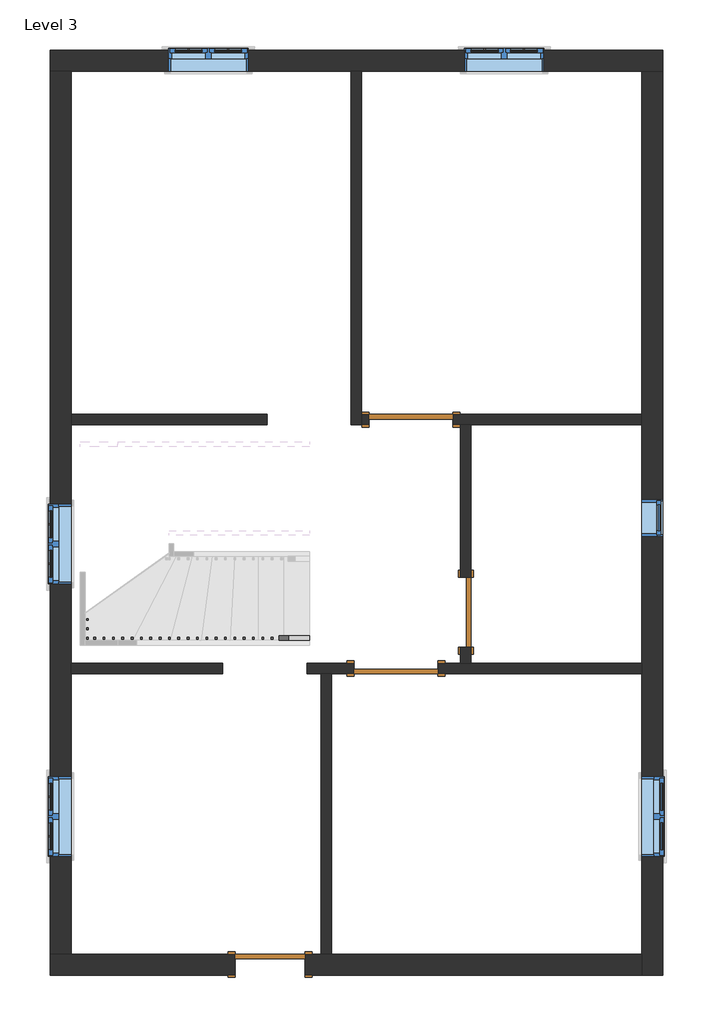
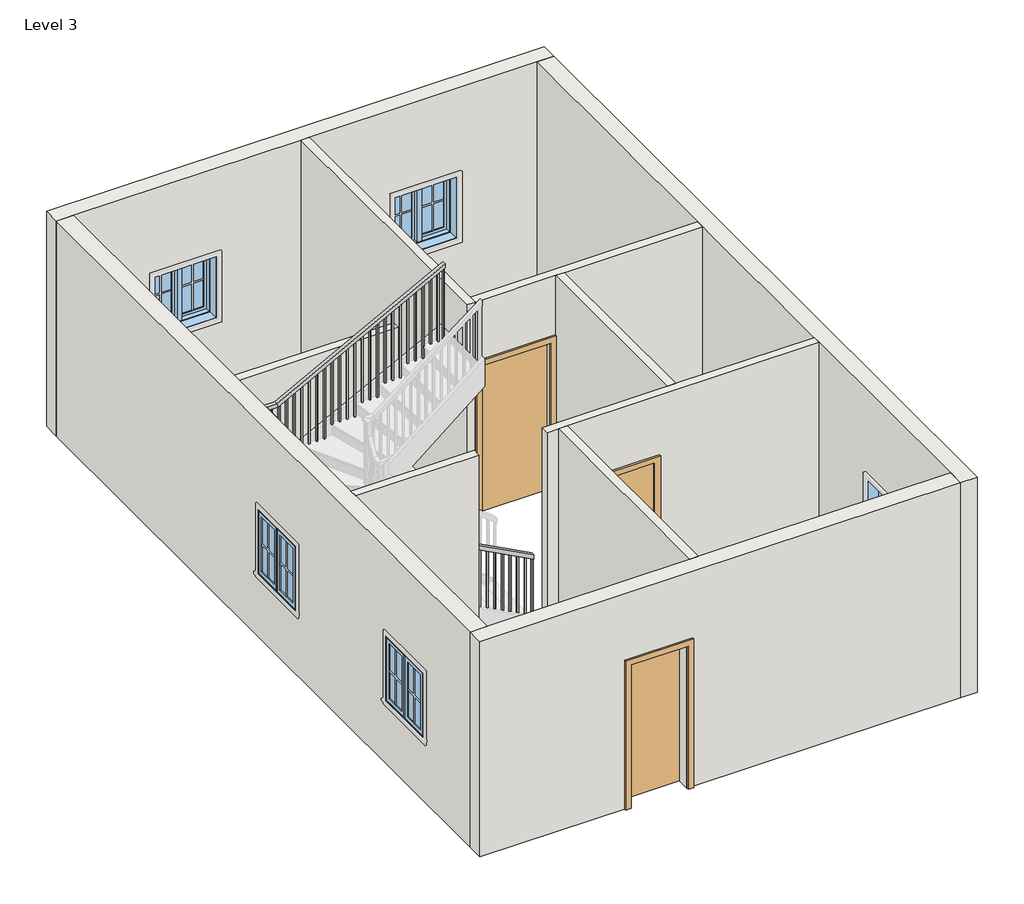
# One storey, part 1 of 2: 11 walls, 6 windows, 4 doors, 1 railing.
"""IFC4 building model written with IfcOpenShell, lengths in millimetres."""

from ifc_helpers import new_model, si_unit, frame, origin, place, context, project, spatial, polyline, outline, extrude, faceted_brep, transform, mapped, element, save
from components import door_d8f5dbb5, door_85036156, door_305aa2a5, door_e5f9f3c4, window_aa618e30, window_339605e1

model = new_model("IFC4")

# Units and contexts
model_context = context("Model", 3, world=origin())
ifc_project = project(units=[si_unit("LENGTHUNIT", "METRE", prefix="MILLI")], contexts=[model_context])

# Site, building, storey
site = spatial("IfcSite", under=ifc_project)
building = spatial("IfcBuilding", under=site)
storey = spatial("IfcBuildingStorey", under=building, Name="Level 3", Elevation=3200.4)

# Doors
placement = place(None, origin())
door_shape = door_d8f5dbb5(model_context)
element("IfcDoor", 1, ObjectType="Single-Flush : 30\" x 80\"", at=placement, inside=storey, context=model_context, shape_type="MappedRepresentation", body=[
    mapped(door_shape, transform((-82.2715692, -955.3070853, 3200.4), x_axis=(0.0, -1.0, 0.0), y_axis=(1.0, 0.0, 0.0), z_axis=(0.0, 0.0, 1.0))),
])
door_2_shape = door_85036156(model_context)
element("IfcDoor", 2, ObjectType="Single-Flush : 30\" x 80\"", at=placement, inside=storey, context=model_context, shape_type="MappedRepresentation", body=[
    mapped(door_2_shape, transform((-2212.5949167, -4784.3570853, 3200.4), x_axis=(-1.0, 0.0, 0.0), y_axis=(0.0, -1.0, 0.0), z_axis=(0.0, 0.0, 1.0))),
])
door_3_shape = door_305aa2a5(model_context)
element("IfcDoor", 3, ObjectType="Single-Flush : 36\" x 84\"", at=placement, inside=storey, context=model_context, shape_type="MappedRepresentation", body=[
    mapped(door_3_shape, transform((-677.5332429, 1140.1929147, 3200.4), x_axis=(-1.0, 0.0, 0.0), y_axis=(0.0, -1.0, 0.0), z_axis=(0.0, 0.0, 1.0))),
])
door_4_shape = door_e5f9f3c4(model_context)
element("IfcDoor", 4, ObjectType="Single-Flush : 36\" x 84\"", at=placement, inside=storey, context=model_context, shape_type="MappedRepresentation", body=[
    mapped(door_4_shape, transform((-842.6332429, -1564.9070853, 3200.4), x_axis=(-1.0, 0.0, 0.0), y_axis=(0.0, -1.0, 0.0), z_axis=(0.0, 0.0, 1.0))),
])

# Railing
element("IfcRailing", 5, ObjectType="Handrail - Rectangular", at=placement, inside=storey, context=model_context, shape_type="SolidModel", body=[
    faceted_brep([(-1783.4132248, -1260.1070853, 4284.1333333), (-1783.4132248, -1260.1070853, 4226.6742652), (-1783.4132248, -1209.3070853, 4226.6742652), (-1783.4132248, -1209.3070853, 4284.1333333), (-4041.1382869, -1260.1070853, 5477.4239201), (-4053.7373514, -1260.1070853, 5426.6239201), (-4053.7373514, -1209.3070853, 5426.6239201), (-4041.1382869, -1209.3070853, 5477.4239201), (-4225.5449167, -1260.1070853, 5477.4239201), (-4225.5449167, -1260.1070853, 5426.6239201), (-4174.7449167, -1209.3070853, 5426.6239201), (-4174.7449167, -1209.3070853, 5477.4239201), (-4225.5449167, -972.7952032, 5477.4239201), (-4225.5449167, -964.8446271, 5426.6239201), (-4174.7449167, -964.8446271, 5426.6239201), (-4174.7449167, -972.7952032, 5477.4239201), (-4225.5449167, 560.7810325, 5969.5094132), (-4225.5449167, 568.7316087, 5918.7094132), (-4174.7449167, 568.7316087, 5918.7094132), (-4174.7449167, 560.7810325, 5969.5094132), (-4225.5449167, 848.0929147, 5969.5094132), (-4225.5449167, 848.0929147, 5918.7094132), (-4174.7449167, 797.2929147, 5918.7094132), (-4174.7449167, 797.2929147, 5969.5094132), (-4041.1382869, 848.0929147, 5969.5094132), (-4028.5392223, 848.0929147, 5918.7094132), (-4028.5392223, 797.2929147, 5918.7094132), (-4041.1382869, 797.2929147, 5969.5094132), (-1783.4132248, 848.0929147, 7162.8), (-1783.4132248, 797.2929147, 7162.8), (-1783.4132248, 797.2929147, 7105.3409318), (-1783.4132248, 848.0929147, 7105.3409318)], [[[0, 1, 2, 3]], [[1, 0, 4, 5]], [[2, 1, 5, 6]], [[3, 2, 6, 7]], [[0, 3, 7, 4]], [[5, 4, 8, 9]], [[6, 5, 9, 10]], [[7, 6, 10, 11]], [[4, 7, 11, 8]], [[9, 8, 12, 13]], [[10, 9, 13, 14]], [[11, 10, 14, 15]], [[8, 11, 15, 12]], [[13, 12, 16, 17]], [[14, 13, 17, 18]], [[15, 14, 18, 19]], [[12, 15, 19, 16]], [[17, 16, 20, 21]], [[18, 17, 21, 22]], [[19, 18, 22, 23]], [[16, 19, 23, 20]], [[21, 20, 24, 25]], [[22, 21, 25, 26]], [[23, 22, 26, 27]], [[20, 23, 27, 24]], [[28, 29, 30, 31]], [[25, 24, 28, 31]], [[26, 25, 31, 30]], [[27, 26, 30, 29]], [[24, 27, 29, 28]]]),
    extrude(outline(polyline([(7058.0597858, -1872.8699167), (6079.0666667, -1872.8699167), (6079.0666667, -1853.8199167), (7068.1284102, -1853.8199167), (7058.0597858, -1872.8699167)])), frame((0.0, 813.1679147, 0.0), z_axis=(0.0, 1.0, 0.0), x_axis=(0.0, 0.0, 1.0)), (0.0, 0.0, 1.0), 19.05),
    extrude(outline(polyline([(7004.3604556, -1974.4699167), (6079.0666667, -1974.4699167), (6079.0666667, -1955.4199167), (7014.42908, -1955.4199167), (7004.3604556, -1974.4699167)])), frame((0.0, 813.1679147, 0.0), z_axis=(0.0, 1.0, 0.0), x_axis=(0.0, 0.0, 1.0)), (0.0, 0.0, 1.0), 19.05),
    extrude(outline(polyline([(6950.6611254, -2076.0699167), (5909.7333333, -2076.0699167), (5909.7333333, -2057.0199167), (6960.7297498, -2057.0199167), (6950.6611254, -2076.0699167)])), frame((0.0, 813.1679147, 0.0), z_axis=(0.0, 1.0, 0.0), x_axis=(0.0, 0.0, 1.0)), (0.0, 0.0, 1.0), 19.05),
    extrude(outline(polyline([(6896.9617952, -2177.6699167), (5909.7333333, -2177.6699167), (5909.7333333, -2158.6199167), (6907.0304196, -2158.6199167), (6896.9617952, -2177.6699167)])), frame((0.0, 813.1679147, 0.0), z_axis=(0.0, 1.0, 0.0), x_axis=(0.0, 0.0, 1.0)), (0.0, 0.0, 1.0), 19.05),
    extrude(outline(polyline([(6843.262465, -2279.2699167), (5909.7333333, -2279.2699167), (5909.7333333, -2260.2199167), (6853.3310894, -2260.2199167), (6843.262465, -2279.2699167)])), frame((0.0, 813.1679147, 0.0), z_axis=(0.0, 1.0, 0.0), x_axis=(0.0, 0.0, 1.0)), (0.0, 0.0, 1.0), 19.05),
    extrude(outline(polyline([(6789.5631348, -2380.8699167), (5740.4, -2380.8699167), (5740.4, -2361.8199167), (6799.6317592, -2361.8199167), (6789.5631348, -2380.8699167)])), frame((0.0, 813.1679147, 0.0), z_axis=(0.0, 1.0, 0.0), x_axis=(0.0, 0.0, 1.0)), (0.0, 0.0, 1.0), 19.05),
    extrude(outline(polyline([(6735.8638046, -2482.4699167), (5740.4, -2482.4699167), (5740.4, -2463.4199167), (6745.932429, -2463.4199167), (6735.8638046, -2482.4699167)])), frame((0.0, 813.1679147, 0.0), z_axis=(0.0, 1.0, 0.0), x_axis=(0.0, 0.0, 1.0)), (0.0, 0.0, 1.0), 19.05),
    extrude(outline(polyline([(6682.1644744, -2584.0699167), (5740.4, -2584.0699167), (5740.4, -2565.0199167), (6692.2330988, -2565.0199167), (6682.1644744, -2584.0699167)])), frame((0.0, 813.1679147, 0.0), z_axis=(0.0, 1.0, 0.0), x_axis=(0.0, 0.0, 1.0)), (0.0, 0.0, 1.0), 19.05),
    extrude(outline(polyline([(6628.4651442, -2685.6699167), (5571.0666667, -2685.6699167), (5571.0666667, -2666.6199167), (6638.5337686, -2666.6199167), (6628.4651442, -2685.6699167)])), frame((0.0, 813.1679147, 0.0), z_axis=(0.0, 1.0, 0.0), x_axis=(0.0, 0.0, 1.0)), (0.0, 0.0, 1.0), 19.05),
    extrude(outline(polyline([(6574.765814, -2787.2699167), (5571.0666667, -2787.2699167), (5571.0666667, -2768.2199167), (6584.8344384, -2768.2199167), (6574.765814, -2787.2699167)])), frame((0.0, 813.1679147, 0.0), z_axis=(0.0, 1.0, 0.0), x_axis=(0.0, 0.0, 1.0)), (0.0, 0.0, 1.0), 19.05),
    extrude(outline(polyline([(6521.0664838, -2888.8699167), (5571.0666667, -2888.8699167), (5571.0666667, -2869.8199167), (6531.1351082, -2869.8199167), (6521.0664838, -2888.8699167)])), frame((0.0, 813.1679147, 0.0), z_axis=(0.0, 1.0, 0.0), x_axis=(0.0, 0.0, 1.0)), (0.0, 0.0, 1.0), 19.05),
    extrude(outline(polyline([(6467.3671536, -2990.4699167), (5401.7333333, -2990.4699167), (5401.7333333, -2971.4199167), (6477.435778, -2971.4199167), (6467.3671536, -2990.4699167)])), frame((0.0, 813.1679147, 0.0), z_axis=(0.0, 1.0, 0.0), x_axis=(0.0, 0.0, 1.0)), (0.0, 0.0, 1.0), 19.05),
    extrude(outline(polyline([(6413.6678234, -3092.0699167), (5401.7333333, -3092.0699167), (5401.7333333, -3073.0199167), (6423.7364478, -3073.0199167), (6413.6678234, -3092.0699167)])), frame((0.0, 813.1679147, 0.0), z_axis=(0.0, 1.0, 0.0), x_axis=(0.0, 0.0, 1.0)), (0.0, 0.0, 1.0), 19.05),
    extrude(outline(polyline([(6359.9684932, -3193.6699167), (5401.7333333, -3193.6699167), (5401.7333333, -3174.6199167), (6370.0371176, -3174.6199167), (6359.9684932, -3193.6699167)])), frame((0.0, 813.1679147, 0.0), z_axis=(0.0, 1.0, 0.0), x_axis=(0.0, 0.0, 1.0)), (0.0, 0.0, 1.0), 19.05),
    extrude(outline(polyline([(6306.269163, -3295.2699167), (5401.7333333, -3295.2699167), (5401.7333333, -3276.2199167), (6316.3377874, -3276.2199167), (6306.269163, -3295.2699167)])), frame((0.0, 813.1679147, 0.0), z_axis=(0.0, 1.0, 0.0), x_axis=(0.0, 0.0, 1.0)), (0.0, 0.0, 1.0), 19.05),
    extrude(outline(polyline([(6252.5698328, -3396.8699167), (5232.4, -3396.8699167), (5232.4, -3377.8199167), (6262.6384572, -3377.8199167), (6252.5698328, -3396.8699167)])), frame((0.0, 813.1679147, 0.0), z_axis=(0.0, 1.0, 0.0), x_axis=(0.0, 0.0, 1.0)), (0.0, 0.0, 1.0), 19.05),
    extrude(outline(polyline([(6198.8705026, -3498.4699167), (5232.4, -3498.4699167), (5232.4, -3479.4199167), (6208.939127, -3479.4199167), (6198.8705026, -3498.4699167)])), frame((0.0, 813.1679147, 0.0), z_axis=(0.0, 1.0, 0.0), x_axis=(0.0, 0.0, 1.0)), (0.0, 0.0, 1.0), 19.05),
    extrude(outline(polyline([(6145.1711724, -3600.0699167), (5232.4, -3600.0699167), (5232.4, -3581.0199167), (6155.2397968, -3581.0199167), (6145.1711724, -3600.0699167)])), frame((0.0, 813.1679147, 0.0), z_axis=(0.0, 1.0, 0.0), x_axis=(0.0, 0.0, 1.0)), (0.0, 0.0, 1.0), 19.05),
    extrude(outline(polyline([(6091.4718422, -3701.6699167), (5232.4, -3701.6699167), (5232.4, -3682.6199167), (6101.5404666, -3682.6199167), (6091.4718422, -3701.6699167)])), frame((0.0, 813.1679147, 0.0), z_axis=(0.0, 1.0, 0.0), x_axis=(0.0, 0.0, 1.0)), (0.0, 0.0, 1.0), 19.05),
    extrude(outline(polyline([(6037.772512, -3803.2699167), (5063.0666667, -3803.2699167), (5063.0666667, -3784.2199167), (6047.8411364, -3784.2199167), (6037.772512, -3803.2699167)])), frame((0.0, 813.1679147, 0.0), z_axis=(0.0, 1.0, 0.0), x_axis=(0.0, 0.0, 1.0)), (0.0, 0.0, 1.0), 19.05),
    extrude(outline(polyline([(5984.0731818, -3904.8699167), (5063.0666667, -3904.8699167), (5063.0666667, -3885.8199167), (5994.1418062, -3885.8199167), (5984.0731818, -3904.8699167)])), frame((0.0, 813.1679147, 0.0), z_axis=(0.0, 1.0, 0.0), x_axis=(0.0, 0.0, 1.0)), (0.0, 0.0, 1.0), 19.05),
    extrude(outline(polyline([(5930.3738516, -4006.4699167), (5063.0666667, -4006.4699167), (5063.0666667, -3987.4199167), (5940.442476, -3987.4199167), (5930.3738516, -4006.4699167)])), frame((0.0, 813.1679147, 0.0), z_axis=(0.0, 1.0, 0.0), x_axis=(0.0, 0.0, 1.0)), (0.0, 0.0, 1.0), 19.05),
    extrude(outline(polyline([(-4108.0699167, 832.2179147), (-4089.0199167, 832.2179147), (-4089.0199167, 813.1679147), (-4108.0699167, 813.1679147), (-4108.0699167, 832.2179147)])), frame((0.0, 0.0, 5063.0666667), z_axis=(0.0, 0.0, 1.0), x_axis=(1.0, 0.0, 0.0)), (0.0, 0.0, 1.0), 855.6427466),
    extrude(outline(polyline([(-4209.6699167, 787.7679147), (-4209.6699167, 806.8179147), (-4190.6199167, 806.8179147), (-4190.6199167, 787.7679147), (-4209.6699167, 787.7679147)])), frame((0.0, 0.0, 5063.0666667), z_axis=(0.0, 0.0, 1.0), x_axis=(1.0, 0.0, 0.0)), (0.0, 0.0, 1.0), 855.6427466),
    extrude(outline(polyline([(-4209.6699167, 686.1679147), (-4209.6699167, 705.2179147), (-4190.6199167, 705.2179147), (-4190.6199167, 686.1679147), (-4209.6699167, 686.1679147)])), frame((0.0, 0.0, 5063.0666667), z_axis=(0.0, 0.0, 1.0), x_axis=(1.0, 0.0, 0.0)), (0.0, 0.0, 1.0), 855.6427466),
    extrude(outline(polyline([(-4209.6699167, 584.5679147), (-4209.6699167, 603.6179147), (-4190.6199167, 603.6179147), (-4190.6199167, 584.5679147), (-4209.6699167, 584.5679147)])), frame((0.0, 0.0, 5063.0666667), z_axis=(0.0, 0.0, 1.0), x_axis=(1.0, 0.0, 0.0)), (0.0, 0.0, 1.0), 855.6427466),
    extrude(outline(polyline([(502.0179147, 5897.3026907), (502.0179147, 4893.7333333), (482.9679147, 4893.7333333), (482.9679147, 5891.1900316), (502.0179147, 5897.3026907)])), frame((-4209.6699167, 0.0, 0.0), z_axis=(1.0, 0.0, 0.0), x_axis=(0.0, 1.0, 0.0)), (0.0, 0.0, 1.0), 19.05),
    extrude(outline(polyline([(400.4179147, 5864.7018425), (400.4179147, 4893.7333333), (381.3679147, 4893.7333333), (381.3679147, 5858.5891834), (400.4179147, 5864.7018425)])), frame((-4209.6699167, 0.0, 0.0), z_axis=(1.0, 0.0, 0.0), x_axis=(0.0, 1.0, 0.0)), (0.0, 0.0, 1.0), 19.05),
    extrude(outline(polyline([(298.8179147, 5832.1009942), (298.8179147, 4893.7333333), (279.7679147, 4893.7333333), (279.7679147, 5825.9883352), (298.8179147, 5832.1009942)])), frame((-4209.6699167, 0.0, 0.0), z_axis=(1.0, 0.0, 0.0), x_axis=(0.0, 1.0, 0.0)), (0.0, 0.0, 1.0), 19.05),
    extrude(outline(polyline([(197.2179147, 5799.500146), (197.2179147, 4893.7333333), (178.1679147, 4893.7333333), (178.1679147, 5793.387487), (197.2179147, 5799.500146)])), frame((-4209.6699167, 0.0, 0.0), z_axis=(1.0, 0.0, 0.0), x_axis=(0.0, 1.0, 0.0)), (0.0, 0.0, 1.0), 19.05),
    extrude(outline(polyline([(95.6179147, 5766.8992978), (95.6179147, 4893.7333333), (76.5679147, 4893.7333333), (76.5679147, 5760.7866387), (95.6179147, 5766.8992978)])), frame((-4209.6699167, 0.0, 0.0), z_axis=(1.0, 0.0, 0.0), x_axis=(0.0, 1.0, 0.0)), (0.0, 0.0, 1.0), 19.05),
    extrude(outline(polyline([(-5.9820853, 5734.2984495), (-5.9820853, 4724.4), (-25.0320853, 4724.4), (-25.0320853, 5728.1857905), (-5.9820853, 5734.2984495)])), frame((-4209.6699167, 0.0, 0.0), z_axis=(1.0, 0.0, 0.0), x_axis=(0.0, 1.0, 0.0)), (0.0, 0.0, 1.0), 19.05),
    extrude(outline(polyline([(-107.5820853, 5701.6976013), (-107.5820853, 4724.4), (-126.6320853, 4724.4), (-126.6320853, 5695.5849423), (-107.5820853, 5701.6976013)])), frame((-4209.6699167, 0.0, 0.0), z_axis=(1.0, 0.0, 0.0), x_axis=(0.0, 1.0, 0.0)), (0.0, 0.0, 1.0), 19.05),
    extrude(outline(polyline([(-209.1820853, 5669.0967531), (-209.1820853, 4724.4), (-228.2320853, 4724.4), (-228.2320853, 5662.984094), (-209.1820853, 5669.0967531)])), frame((-4209.6699167, 0.0, 0.0), z_axis=(1.0, 0.0, 0.0), x_axis=(0.0, 1.0, 0.0)), (0.0, 0.0, 1.0), 19.05),
    extrude(outline(polyline([(-310.7820853, 5636.4959049), (-310.7820853, 4724.4), (-329.8320853, 4724.4), (-329.8320853, 5630.3832458), (-310.7820853, 5636.4959049)])), frame((-4209.6699167, 0.0, 0.0), z_axis=(1.0, 0.0, 0.0), x_axis=(0.0, 1.0, 0.0)), (0.0, 0.0, 1.0), 19.05),
    extrude(outline(polyline([(-412.3820853, 5603.8950566), (-412.3820853, 4724.4), (-431.4320853, 4724.4), (-431.4320853, 5597.7823976), (-412.3820853, 5603.8950566)])), frame((-4209.6699167, 0.0, 0.0), z_axis=(1.0, 0.0, 0.0), x_axis=(0.0, 1.0, 0.0)), (0.0, 0.0, 1.0), 19.05),
    extrude(outline(polyline([(-513.9820853, 5571.2942084), (-513.9820853, 4555.0666667), (-533.0320853, 4555.0666667), (-533.0320853, 5565.1815494), (-513.9820853, 5571.2942084)])), frame((-4209.6699167, 0.0, 0.0), z_axis=(1.0, 0.0, 0.0), x_axis=(0.0, 1.0, 0.0)), (0.0, 0.0, 1.0), 19.05),
    extrude(outline(polyline([(-615.5820853, 5538.6933602), (-615.5820853, 4555.0666667), (-634.6320853, 4555.0666667), (-634.6320853, 5532.5807011), (-615.5820853, 5538.6933602)])), frame((-4209.6699167, 0.0, 0.0), z_axis=(1.0, 0.0, 0.0), x_axis=(0.0, 1.0, 0.0)), (0.0, 0.0, 1.0), 19.05),
    extrude(outline(polyline([(-717.1820853, 5506.092512), (-717.1820853, 4555.0666667), (-736.2320853, 4555.0666667), (-736.2320853, 5499.9798529), (-717.1820853, 5506.092512)])), frame((-4209.6699167, 0.0, 0.0), z_axis=(1.0, 0.0, 0.0), x_axis=(0.0, 1.0, 0.0)), (0.0, 0.0, 1.0), 19.05),
    extrude(outline(polyline([(-818.7820853, 5473.4916637), (-818.7820853, 4555.0666667), (-837.8320853, 4555.0666667), (-837.8320853, 5467.3790047), (-818.7820853, 5473.4916637)])), frame((-4209.6699167, 0.0, 0.0), z_axis=(1.0, 0.0, 0.0), x_axis=(0.0, 1.0, 0.0)), (0.0, 0.0, 1.0), 19.05),
    extrude(outline(polyline([(-920.3820853, 5440.8908155), (-920.3820853, 4555.0666667), (-939.4320853, 4555.0666667), (-939.4320853, 5434.7781565), (-920.3820853, 5440.8908155)])), frame((-4209.6699167, 0.0, 0.0), z_axis=(1.0, 0.0, 0.0), x_axis=(0.0, 1.0, 0.0)), (0.0, 0.0, 1.0), 19.05),
    extrude(outline(polyline([(-4209.6699167, -1041.0320853), (-4209.6699167, -1021.9820853), (-4190.6199167, -1021.9820853), (-4190.6199167, -1041.0320853), (-4209.6699167, -1041.0320853)])), frame((0.0, 0.0, 4385.7333333), z_axis=(0.0, 0.0, 1.0), x_axis=(1.0, 0.0, 0.0)), (0.0, 0.0, 1.0), 1040.8905868),
    extrude(outline(polyline([(-4209.6699167, -1142.6320853), (-4209.6699167, -1123.5820853), (-4190.6199167, -1123.5820853), (-4190.6199167, -1142.6320853), (-4209.6699167, -1142.6320853)])), frame((0.0, 0.0, 4385.7333333), z_axis=(0.0, 0.0, 1.0), x_axis=(1.0, 0.0, 0.0)), (0.0, 0.0, 1.0), 1040.8905868),
    extrude(outline(polyline([(-4110.6882248, -1244.2320853), (-4129.7382248, -1244.2320853), (-4129.7382248, -1225.1820853), (-4110.6882248, -1225.1820853), (-4110.6882248, -1244.2320853)])), frame((0.0, 0.0, 4385.7333333), z_axis=(0.0, 0.0, 1.0), x_axis=(1.0, 0.0, 0.0)), (0.0, 0.0, 1.0), 1040.8905868),
    extrude(outline(polyline([(5413.0938418, -4028.1382248), (4385.7333333, -4028.1382248), (4385.7333333, -4009.0882248), (5403.0252174, -4009.0882248), (5413.0938418, -4028.1382248)])), frame((0.0, -1244.2320853, 0.0), z_axis=(0.0, 1.0, 0.0), x_axis=(0.0, 0.0, 1.0)), (0.0, 0.0, 1.0), 19.05),
    extrude(outline(polyline([(5359.3945116, -3926.5382248), (4385.7333333, -3926.5382248), (4385.7333333, -3907.4882248), (5349.3258872, -3907.4882248), (5359.3945116, -3926.5382248)])), frame((0.0, -1244.2320853, 0.0), z_axis=(0.0, 1.0, 0.0), x_axis=(0.0, 0.0, 1.0)), (0.0, 0.0, 1.0), 19.05),
    extrude(outline(polyline([(5305.6951814, -3824.9382248), (4385.7333333, -3824.9382248), (4385.7333333, -3805.8882248), (5295.626557, -3805.8882248), (5305.6951814, -3824.9382248)])), frame((0.0, -1244.2320853, 0.0), z_axis=(0.0, 1.0, 0.0), x_axis=(0.0, 0.0, 1.0)), (0.0, 0.0, 1.0), 19.05),
    extrude(outline(polyline([(5251.9958512, -3723.3382248), (4385.7333333, -3723.3382248), (4385.7333333, -3704.2882248), (5241.9272268, -3704.2882248), (5251.9958512, -3723.3382248)])), frame((0.0, -1244.2320853, 0.0), z_axis=(0.0, 1.0, 0.0), x_axis=(0.0, 0.0, 1.0)), (0.0, 0.0, 1.0), 19.05),
    extrude(outline(polyline([(5198.296521, -3621.7382248), (4216.4, -3621.7382248), (4216.4, -3602.6882248), (5188.2278966, -3602.6882248), (5198.296521, -3621.7382248)])), frame((0.0, -1244.2320853, 0.0), z_axis=(0.0, 1.0, 0.0), x_axis=(0.0, 0.0, 1.0)), (0.0, 0.0, 1.0), 19.05),
    extrude(outline(polyline([(5144.5971908, -3520.1382248), (4216.4, -3520.1382248), (4216.4, -3501.0882248), (5134.5285664, -3501.0882248), (5144.5971908, -3520.1382248)])), frame((0.0, -1244.2320853, 0.0), z_axis=(0.0, 1.0, 0.0), x_axis=(0.0, 0.0, 1.0)), (0.0, 0.0, 1.0), 19.05),
    extrude(outline(polyline([(5090.8978606, -3418.5382248), (4216.4, -3418.5382248), (4216.4, -3399.4882248), (5080.8292362, -3399.4882248), (5090.8978606, -3418.5382248)])), frame((0.0, -1244.2320853, 0.0), z_axis=(0.0, 1.0, 0.0), x_axis=(0.0, 0.0, 1.0)), (0.0, 0.0, 1.0), 19.05),
    extrude(outline(polyline([(5037.1985304, -3316.9382248), (4216.4, -3316.9382248), (4216.4, -3297.8882248), (5027.129906, -3297.8882248), (5037.1985304, -3316.9382248)])), frame((0.0, -1244.2320853, 0.0), z_axis=(0.0, 1.0, 0.0), x_axis=(0.0, 0.0, 1.0)), (0.0, 0.0, 1.0), 19.05),
    extrude(outline(polyline([(4983.4992002, -3215.3382248), (4047.0666667, -3215.3382248), (4047.0666667, -3196.2882248), (4973.4305758, -3196.2882248), (4983.4992002, -3215.3382248)])), frame((0.0, -1244.2320853, 0.0), z_axis=(0.0, 1.0, 0.0), x_axis=(0.0, 0.0, 1.0)), (0.0, 0.0, 1.0), 19.05),
    extrude(outline(polyline([(4929.79987, -3113.7382248), (4047.0666667, -3113.7382248), (4047.0666667, -3094.6882248), (4919.7312456, -3094.6882248), (4929.79987, -3113.7382248)])), frame((0.0, -1244.2320853, 0.0), z_axis=(0.0, 1.0, 0.0), x_axis=(0.0, 0.0, 1.0)), (0.0, 0.0, 1.0), 19.05),
    extrude(outline(polyline([(4876.1005398, -3012.1382248), (4047.0666667, -3012.1382248), (4047.0666667, -2993.0882248), (4866.0319154, -2993.0882248), (4876.1005398, -3012.1382248)])), frame((0.0, -1244.2320853, 0.0), z_axis=(0.0, 1.0, 0.0), x_axis=(0.0, 0.0, 1.0)), (0.0, 0.0, 1.0), 19.05),
    extrude(outline(polyline([(4822.4012096, -2910.5382248), (3877.7333333, -2910.5382248), (3877.7333333, -2891.4882248), (4812.3325852, -2891.4882248), (4822.4012096, -2910.5382248)])), frame((0.0, -1244.2320853, 0.0), z_axis=(0.0, 1.0, 0.0), x_axis=(0.0, 0.0, 1.0)), (0.0, 0.0, 1.0), 19.05),
    extrude(outline(polyline([(4768.7018794, -2808.9382248), (3877.7333333, -2808.9382248), (3877.7333333, -2789.8882248), (4758.633255, -2789.8882248), (4768.7018794, -2808.9382248)])), frame((0.0, -1244.2320853, 0.0), z_axis=(0.0, 1.0, 0.0), x_axis=(0.0, 0.0, 1.0)), (0.0, 0.0, 1.0), 19.05),
    extrude(outline(polyline([(4715.0025492, -2707.3382248), (3877.7333333, -2707.3382248), (3877.7333333, -2688.2882248), (4704.9339248, -2688.2882248), (4715.0025492, -2707.3382248)])), frame((0.0, -1244.2320853, 0.0), z_axis=(0.0, 1.0, 0.0), x_axis=(0.0, 0.0, 1.0)), (0.0, 0.0, 1.0), 19.05),
    extrude(outline(polyline([(4661.303219, -2605.7382248), (3708.4, -2605.7382248), (3708.4, -2586.6882248), (4651.2345946, -2586.6882248), (4661.303219, -2605.7382248)])), frame((0.0, -1244.2320853, 0.0), z_axis=(0.0, 1.0, 0.0), x_axis=(0.0, 0.0, 1.0)), (0.0, 0.0, 1.0), 19.05),
    extrude(outline(polyline([(4607.6038888, -2504.1382248), (3708.4, -2504.1382248), (3708.4, -2485.0882248), (4597.5352644, -2485.0882248), (4607.6038888, -2504.1382248)])), frame((0.0, -1244.2320853, 0.0), z_axis=(0.0, 1.0, 0.0), x_axis=(0.0, 0.0, 1.0)), (0.0, 0.0, 1.0), 19.05),
    extrude(outline(polyline([(4553.9045586, -2402.5382248), (3708.4, -2402.5382248), (3708.4, -2383.4882248), (4543.8359342, -2383.4882248), (4553.9045586, -2402.5382248)])), frame((0.0, -1244.2320853, 0.0), z_axis=(0.0, 1.0, 0.0), x_axis=(0.0, 0.0, 1.0)), (0.0, 0.0, 1.0), 19.05),
    extrude(outline(polyline([(4500.2052284, -2300.9382248), (3539.0666667, -2300.9382248), (3539.0666667, -2281.8882248), (4490.136604, -2281.8882248), (4500.2052284, -2300.9382248)])), frame((0.0, -1244.2320853, 0.0), z_axis=(0.0, 1.0, 0.0), x_axis=(0.0, 0.0, 1.0)), (0.0, 0.0, 1.0), 19.05),
    extrude(outline(polyline([(4446.5058982, -2199.3382248), (3539.0666667, -2199.3382248), (3539.0666667, -2180.2882248), (4436.4372738, -2180.2882248), (4446.5058982, -2199.3382248)])), frame((0.0, -1244.2320853, 0.0), z_axis=(0.0, 1.0, 0.0), x_axis=(0.0, 0.0, 1.0)), (0.0, 0.0, 1.0), 19.05),
    extrude(outline(polyline([(4392.806568, -2097.7382248), (3539.0666667, -2097.7382248), (3539.0666667, -2078.6882248), (4382.7379436, -2078.6882248), (4392.806568, -2097.7382248)])), frame((0.0, -1244.2320853, 0.0), z_axis=(0.0, 1.0, 0.0), x_axis=(0.0, 0.0, 1.0)), (0.0, 0.0, 1.0), 19.05),
    extrude(outline(polyline([(4339.1072378, -1996.1382248), (3369.7333333, -1996.1382248), (3369.7333333, -1977.0882248), (4329.0386134, -1977.0882248), (4339.1072378, -1996.1382248)])), frame((0.0, -1244.2320853, 0.0), z_axis=(0.0, 1.0, 0.0), x_axis=(0.0, 0.0, 1.0)), (0.0, 0.0, 1.0), 19.05),
    extrude(outline(polyline([(4285.4079076, -1894.5382248), (3369.7333333, -1894.5382248), (3369.7333333, -1875.4882248), (4275.3392831, -1875.4882248), (4285.4079076, -1894.5382248)])), frame((0.0, -1244.2320853, 0.0), z_axis=(0.0, 1.0, 0.0), x_axis=(0.0, 0.0, 1.0)), (0.0, 0.0, 1.0), 19.05),
    extrude(outline(polyline([(-4209.6699167, 813.1679147), (-4209.6699167, 832.2179147), (-4190.6199167, 832.2179147), (-4190.6199167, 813.1679147), (-4209.6699167, 813.1679147)])), frame((0.0, 0.0, 5063.0666667), z_axis=(0.0, 0.0, 1.0), x_axis=(1.0, 0.0, 0.0)), (0.0, 0.0, 1.0), 855.6427466),
    extrude(outline(polyline([(-4190.6199167, -1244.2320853), (-4209.6699167, -1244.2320853), (-4209.6699167, -1225.1820853), (-4190.6199167, -1225.1820853), (-4190.6199167, -1244.2320853)])), frame((0.0, 0.0, 4385.7333333), z_axis=(0.0, 0.0, 1.0), x_axis=(1.0, 0.0, 0.0)), (0.0, 0.0, 1.0), 1040.8905868),
    extrude(outline(polyline([(7095.2723074, -1802.4632248), (6079.0666667, -1802.4632248), (6079.0666667, -1783.4132248), (7105.3409318, -1783.4132248), (7095.2723074, -1802.4632248)])), frame((0.0, 813.1679147, 0.0), z_axis=(0.0, 1.0, 0.0), x_axis=(0.0, 0.0, 1.0)), (0.0, 0.0, 1.0), 19.05),
    extrude(outline(polyline([(4236.7428896, -1802.4632248), (3369.7333333, -1802.4632248), (3369.7333333, -1783.4132248), (4226.6742652, -1783.4132248), (4236.7428896, -1802.4632248)])), frame((0.0, -1244.2320853, 0.0), z_axis=(0.0, 1.0, 0.0), x_axis=(0.0, 0.0, 1.0)), (0.0, 0.0, 1.0), 19.05),
])

# Walls
element("IfcWall", 6, ObjectType="WALL4.5\"", at=placement, inside=storey, context=model_context, shape_type="Brep", body=[
    faceted_brep([(-1329.9449167, 4931.1429147, 3200.4), (-1329.9449167, 1083.0429147, 3200.4), (-1329.9449167, 1083.0429147, 6248.4), (-1329.9449167, 4931.1429147, 6248.4), (-1215.6449167, 4931.1429147, 3200.4), (-1215.6449167, 4931.1429147, 6248.4), (-1215.6449167, 1197.3429147, 6248.4), (-1215.6449167, 1083.0429147, 6248.4), (-1215.6449167, 1083.0429147, 3200.4), (-1215.6449167, 1197.3429147, 3200.4)], [[[0, 1, 2, 3]], [[4, 5, 6, 7, 8, 9]], [[1, 0, 4, 9, 8]], [[0, 3, 5, 4]], [[2, 1, 8, 7]], [[3, 2, 7, 6, 5]]]),
])
element("IfcWall", 7, ObjectType="WALL4.5\"", at=placement, inside=storey, context=model_context, shape_type="Brep", body=[
    faceted_brep([(-1215.6449167, 1083.0429147, 3200.4), (-1134.7332429, 1083.0429147, 3200.4), (-1134.7332429, 1083.0429147, 5334.0), (-220.3332429, 1083.0429147, 5334.0), (-220.3332429, 1083.0429147, 3200.4), (-139.4215692, 1083.0429147, 3200.4), (-25.1215692, 1083.0429147, 3200.4), (1832.3550833, 1083.0429147, 3200.4), (1832.3550833, 1083.0429147, 6248.4), (-25.1215692, 1083.0429147, 6248.4), (-139.4215692, 1083.0429147, 6248.4), (-1215.6449167, 1083.0429147, 6248.4), (-1134.7332429, 1197.3429147, 5334.0), (-1134.7332429, 1197.3429147, 3200.4), (-1215.6449167, 1197.3429147, 3200.4), (-1215.6449167, 1197.3429147, 6248.4), (1832.3550833, 1197.3429147, 6248.4), (1832.3550833, 1197.3429147, 3200.4), (-220.3332429, 1197.3429147, 3200.4), (-220.3332429, 1197.3429147, 5334.0)], [[[0, 1, 2, 3, 4, 5, 6, 7, 8, 9, 10, 11]], [[12, 13, 14, 15, 16, 17, 18, 19]], [[18, 17, 7, 6, 5, 4]], [[14, 13, 1, 0]], [[0, 11, 15, 14]], [[8, 7, 17, 16]], [[2, 1, 13, 12]], [[3, 2, 12, 19]], [[4, 3, 19, 18]], [[11, 10, 9, 8, 16, 15]]]),
])
element("IfcWall", 8, ObjectType="WALL4.5\"", at=placement, inside=storey, context=model_context, shape_type="SweptSolid", body=[
    extrude(outline(polyline([(-2244.3449167, 1083.0429147), (-4377.9449167, 1083.0429147), (-4377.9449167, 1197.3429147), (-2244.3449167, 1197.3429147), (-2244.3449167, 1083.0429147)])), frame((0.0, 0.0, 3200.4), z_axis=(0.0, 0.0, 1.0), x_axis=(1.0, 0.0, 0.0)), (0.0, 0.0, 1.0), 3048.0),
])
element("IfcWall", 9, ObjectType="WALL4.5\"", at=placement, inside=storey, context=model_context, shape_type="SweptSolid", body=[
    extrude(outline(polyline([(-1336.3070853, 5232.4), (-1336.3070853, 3200.4), (-1507.7570853, 3200.4), (-1507.7570853, 6248.4), (1083.0429147, 6248.4), (1083.0429147, 3200.4), (-574.3070853, 3200.4), (-574.3070853, 5232.4), (-1336.3070853, 5232.4)])), frame((-139.4215692, 0.0, 0.0), z_axis=(1.0, 0.0, 0.0), x_axis=(0.0, 1.0, 0.0)), (0.0, 0.0, 1.0), 114.3),
])
element("IfcWall", 10, ObjectType="WALL4.5\"", at=placement, inside=storey, context=model_context, shape_type="SweptSolid", body=[
    extrude(outline(polyline([(-2726.9449167, -1622.0570853), (-4377.9449167, -1622.0570853), (-4377.9449167, -1507.7570853), (-2726.9449167, -1507.7570853), (-2726.9449167, -1622.0570853)])), frame((0.0, 0.0, 3200.4), z_axis=(0.0, 0.0, 1.0), x_axis=(1.0, 0.0, 0.0)), (0.0, 0.0, 1.0), 3048.0),
])
element("IfcWall", 11, ObjectType="WALL4.5\"", at=placement, inside=storey, context=model_context, shape_type="Brep", body=[
    faceted_brep([(-1812.5449167, -1622.0570853, 3200.4), (-1660.1449167, -1622.0570853, 3200.4), (-1545.8449167, -1622.0570853, 3200.4), (-1299.8332429, -1622.0570853, 3200.4), (-1299.8332429, -1622.0570853, 5334.0), (-385.4332429, -1622.0570853, 5334.0), (-385.4332429, -1622.0570853, 3200.4), (1832.3550833, -1622.0570853, 3200.4), (1832.3550833, -1622.0570853, 6248.4), (-1545.8449167, -1622.0570853, 6248.4), (-1660.1449167, -1622.0570853, 6248.4), (-1812.5449167, -1622.0570853, 6248.4), (-1299.8332429, -1507.7570853, 5334.0), (-1299.8332429, -1507.7570853, 3200.4), (-1812.5449167, -1507.7570853, 3200.4), (-1812.5449167, -1507.7570853, 6248.4), (-139.4215692, -1507.7570853, 6248.4), (-25.1215692, -1507.7570853, 6248.4), (1832.3550833, -1507.7570853, 6248.4), (1832.3550833, -1507.7570853, 3200.4), (-25.1215692, -1507.7570853, 3200.4), (-139.4215692, -1507.7570853, 3200.4), (-385.4332429, -1507.7570853, 3200.4), (-385.4332429, -1507.7570853, 5334.0)], [[[0, 1, 2, 3, 4, 5, 6, 7, 8, 9, 10, 11]], [[12, 13, 14, 15, 16, 17, 18, 19, 20, 21, 22, 23]], [[14, 13, 3, 2, 1, 0]], [[22, 21, 20, 19, 7, 6]], [[0, 11, 15, 14]], [[8, 7, 19, 18]], [[4, 3, 13, 12]], [[5, 4, 12, 23]], [[6, 5, 23, 22]], [[11, 10, 9, 8, 18, 17, 16, 15]]]),
])
element("IfcWall", 12, ObjectType="WALL4.5\"", at=placement, inside=storey, context=model_context, shape_type="SweptSolid", body=[
    extrude(outline(polyline([(-1660.1449167, -4670.0570853), (-1660.1449167, -1622.0570853), (-1545.8449167, -1622.0570853), (-1545.8449167, -4670.0570853), (-1660.1449167, -4670.0570853)])), frame((0.0, 0.0, 3200.4), z_axis=(0.0, 0.0, 1.0), x_axis=(1.0, 0.0, 0.0)), (0.0, 0.0, 1.0), 3048.0),
])
element("IfcWall", 13, ObjectType="WALL9\"", at=placement, inside=storey, context=model_context, shape_type="Brep", body=[
    faceted_brep([(-4606.5449167, 4931.1429147, 3200.4), (-4377.9449167, 4931.1429147, 3200.4), (-1329.9449167, 4931.1429147, 3200.4), (-1215.6449167, 4931.1429147, 3200.4), (1832.3550833, 4931.1429147, 3200.4), (2060.9550833, 4931.1429147, 3200.4), (2060.9550833, 4931.1429147, 6248.4), (1832.3550833, 4931.1429147, 6248.4), (-1215.6449167, 4931.1429147, 6248.4), (-1329.9449167, 4931.1429147, 6248.4), (-4377.9449167, 4931.1429147, 6248.4), (-4606.5449167, 4931.1429147, 6248.4), (-2450.7199167, 4931.1429147, 5029.2), (-2450.7199167, 4931.1429147, 4114.8), (-3314.3199167, 4931.1429147, 4114.8), (-3314.3199167, 4931.1429147, 5029.2), (768.7300833, 4931.1429147, 5029.2), (768.7300833, 4931.1429147, 4114.8), (-94.8699167, 4931.1429147, 4114.8), (-94.8699167, 4931.1429147, 5029.2), (-4606.5449167, 5159.7429147, 3200.4), (-4606.5449167, 5159.7429147, 6248.4), (2060.9550833, 5159.7429147, 6248.4), (2060.9550833, 5159.7429147, 3200.4), (-2450.7199167, 5159.7429147, 5029.2), (-3314.3199167, 5159.7429147, 5029.2), (-3314.3199167, 5159.7429147, 4114.8), (-2450.7199167, 5159.7429147, 4114.8), (768.7300833, 5159.7429147, 5029.2), (-94.8699167, 5159.7429147, 5029.2), (-94.8699167, 5159.7429147, 4114.8), (768.7300833, 5159.7429147, 4114.8)], [[[0, 1, 2, 3, 4, 5, 6, 7, 8, 9, 10, 11], [12, 13, 14, 15], [16, 17, 18, 19]], [[20, 21, 22, 23], [24, 25, 26, 27], [28, 29, 30, 31]], [[5, 4, 3, 2, 1, 0, 20, 23]], [[6, 5, 23, 22]], [[0, 11, 21, 20]], [[13, 12, 24, 27]], [[14, 13, 27, 26]], [[15, 14, 26, 25]], [[12, 15, 25, 24]], [[17, 16, 28, 31]], [[18, 17, 31, 30]], [[19, 18, 30, 29]], [[16, 19, 29, 28]], [[11, 10, 9, 8, 7, 6, 22, 21]]]),
])
element("IfcWall", 14, ObjectType="WALL9\"", at=placement, inside=storey, context=model_context, shape_type="Brep", body=[
    faceted_brep([(1832.3550833, 4931.1429147, 3200.4), (1832.3550833, 1197.3429147, 3200.4), (1832.3550833, 1083.0429147, 3200.4), (1832.3550833, -1507.7570853, 3200.4), (1832.3550833, -1622.0570853, 3200.4), (1832.3550833, -4670.0570853, 3200.4), (1832.3550833, -4898.6570853, 3200.4), (1832.3550833, -4898.6570853, 6248.4), (1832.3550833, -4670.0570853, 6248.4), (1832.3550833, -1622.0570853, 6248.4), (1832.3550833, -1507.7570853, 6248.4), (1832.3550833, 1083.0429147, 6248.4), (1832.3550833, 1197.3429147, 6248.4), (1832.3550833, 4931.1429147, 6248.4), (1832.3550833, -129.8070853, 4724.4), (1832.3550833, -129.8070853, 4114.8), (1832.3550833, 276.5929147, 4114.8), (1832.3550833, 276.5929147, 4724.4), (1832.3550833, -3606.4320853, 5029.2), (1832.3550833, -3606.4320853, 4114.8), (1832.3550833, -2742.8320853, 4114.8), (1832.3550833, -2742.8320853, 5029.2), (2060.9550833, 4931.1429147, 3200.4), (2060.9550833, 4931.1429147, 6248.4), (2060.9550833, -4898.6570853, 6248.4), (2060.9550833, -4898.6570853, 3200.4), (2060.9550833, -129.8070853, 4724.4), (2060.9550833, 276.5929147, 4724.4), (2060.9550833, 276.5929147, 4114.8), (2060.9550833, -129.8070853, 4114.8), (2060.9550833, -3606.4320853, 5029.2), (2060.9550833, -2742.8320853, 5029.2), (2060.9550833, -2742.8320853, 4114.8), (2060.9550833, -3606.4320853, 4114.8)], [[[0, 1, 2, 3, 4, 5, 6, 7, 8, 9, 10, 11, 12, 13], [14, 15, 16, 17], [18, 19, 20, 21]], [[22, 23, 24, 25], [26, 27, 28, 29], [30, 31, 32, 33]], [[6, 5, 4, 3, 2, 1, 0, 22, 25]], [[0, 13, 23, 22]], [[7, 6, 25, 24]], [[15, 14, 26, 29]], [[16, 15, 29, 28]], [[17, 16, 28, 27]], [[14, 17, 27, 26]], [[19, 18, 30, 33]], [[20, 19, 33, 32]], [[21, 20, 32, 31]], [[18, 21, 31, 30]], [[13, 12, 11, 10, 9, 8, 7, 24, 23]]]),
])
element("IfcWall", 15, ObjectType="WALL9\"", at=placement, inside=storey, context=model_context, shape_type="Brep", body=[
    faceted_brep([(-2593.5949167, -4670.0570853, 5232.4), (-2593.5949167, -4670.0570853, 3200.4), (-4377.9449167, -4670.0570853, 3200.4), (-4606.5449167, -4670.0570853, 3200.4), (-4606.5449167, -4670.0570853, 6248.4), (-4377.9449167, -4670.0570853, 6248.4), (-1660.1449167, -4670.0570853, 6248.4), (-1545.8449167, -4670.0570853, 6248.4), (1832.3550833, -4670.0570853, 6248.4), (1832.3550833, -4670.0570853, 3200.4), (-1545.8449167, -4670.0570853, 3200.4), (-1660.1449167, -4670.0570853, 3200.4), (-1831.5949167, -4670.0570853, 3200.4), (-1831.5949167, -4670.0570853, 5232.4), (-4606.5449167, -4898.6570853, 3200.4), (-2593.5949167, -4898.6570853, 3200.4), (-2593.5949167, -4898.6570853, 5232.4), (-1831.5949167, -4898.6570853, 5232.4), (-1831.5949167, -4898.6570853, 3200.4), (1832.3550833, -4898.6570853, 3200.4), (1832.3550833, -4898.6570853, 6248.4), (-4606.5449167, -4898.6570853, 6248.4)], [[[0, 1, 2, 3, 4, 5, 6, 7, 8, 9, 10, 11, 12, 13]], [[14, 15, 16, 17, 18, 19, 20, 21]], [[3, 2, 1, 15, 14]], [[12, 11, 10, 9, 19, 18]], [[9, 8, 20, 19]], [[4, 3, 14, 21]], [[16, 15, 1, 0]], [[17, 16, 0, 13]], [[18, 17, 13, 12]], [[8, 7, 6, 5, 4, 21, 20]]]),
])
element("IfcWall", 16, ObjectType="WALL9\"", at=placement, inside=storey, context=model_context, shape_type="Brep", body=[
    faceted_brep([(-4377.9449167, -4670.0570853, 3200.4), (-4377.9449167, -1622.0570853, 3200.4), (-4377.9449167, -1507.7570853, 3200.4), (-4377.9449167, 1083.0429147, 3200.4), (-4377.9449167, 1197.3429147, 3200.4), (-4377.9449167, 4931.1429147, 3200.4), (-4377.9449167, 4931.1429147, 6248.4), (-4377.9449167, 1197.3429147, 6248.4), (-4377.9449167, 1083.0429147, 6248.4), (-4377.9449167, -1507.7570853, 6248.4), (-4377.9449167, -1622.0570853, 6248.4), (-4377.9449167, -4670.0570853, 6248.4), (-4377.9449167, -2742.8320853, 5029.2), (-4377.9449167, -2742.8320853, 4114.8), (-4377.9449167, -3606.4320853, 4114.8), (-4377.9449167, -3606.4320853, 5029.2), (-4377.9449167, 219.4429147, 5029.2), (-4377.9449167, 219.4429147, 4114.8), (-4377.9449167, -644.1570853, 4114.8), (-4377.9449167, -644.1570853, 5029.2), (-4606.5449167, -4670.0570853, 3200.4), (-4606.5449167, -4670.0570853, 6248.4), (-4606.5449167, 4931.1429147, 6248.4), (-4606.5449167, 4931.1429147, 3200.4), (-4606.5449167, -2742.8320853, 5029.2), (-4606.5449167, -3606.4320853, 5029.2), (-4606.5449167, -3606.4320853, 4114.8), (-4606.5449167, -2742.8320853, 4114.8), (-4606.5449167, 219.4429147, 5029.2), (-4606.5449167, -644.1570853, 5029.2), (-4606.5449167, -644.1570853, 4114.8), (-4606.5449167, 219.4429147, 4114.8)], [[[0, 1, 2, 3, 4, 5, 6, 7, 8, 9, 10, 11], [12, 13, 14, 15], [16, 17, 18, 19]], [[20, 21, 22, 23], [24, 25, 26, 27], [28, 29, 30, 31]], [[5, 4, 3, 2, 1, 0, 20, 23]], [[0, 11, 21, 20]], [[6, 5, 23, 22]], [[13, 12, 24, 27]], [[14, 13, 27, 26]], [[15, 14, 26, 25]], [[12, 15, 25, 24]], [[17, 16, 28, 31]], [[18, 17, 31, 30]], [[19, 18, 30, 29]], [[16, 19, 29, 28]], [[11, 10, 9, 8, 7, 6, 22, 21]]]),
])

# Windows
window_shape = window_aa618e30(model_context)
element("IfcWindow", 17, ObjectType="Fixed : 16\" x 24\"", at=placement, inside=storey, context=model_context, shape_type="MappedRepresentation", body=[
    mapped(window_shape, transform((1946.6550833, 35.2929147, 3200.4), x_axis=(0.0, -1.0, 0.0), y_axis=(1.0, 0.0, 0.0), z_axis=(0.0, 0.0, 1.0))),
])
window_2_shape = window_339605e1(model_context)
element("IfcWindow", 18, ObjectType="Window-Casement-Double : 34\" x 36\"", at=placement, inside=storey, context=model_context, shape_type="MappedRepresentation", body=[
    mapped(window_2_shape, transform((-2882.5199167, 5045.4429147, 3200.4), x_axis=(1.0, 0.0, 0.0), y_axis=(0.0, 1.0, 0.0), z_axis=(0.0, 0.0, 1.0))),
])
element("IfcWindow", 19, ObjectType="Window-Casement-Double : 34\" x 36\"", at=placement, inside=storey, context=model_context, shape_type="MappedRepresentation", body=[
    mapped(window_2_shape, transform((336.9300833, 5045.4429147, 3200.4), x_axis=(1.0, 0.0, 0.0), y_axis=(0.0, 1.0, 0.0), z_axis=(0.0, 0.0, 1.0))),
])
element("IfcWindow", 20, ObjectType="Window-Casement-Double : 34\" x 36\"", at=placement, inside=storey, context=model_context, shape_type="MappedRepresentation", body=[
    mapped(window_2_shape, transform((1946.6550833, -3174.6320853, 3200.4), x_axis=(0.0, -1.0, 0.0), y_axis=(1.0, 0.0, 0.0), z_axis=(0.0, 0.0, 1.0))),
])
element("IfcWindow", 21, ObjectType="Window-Casement-Double : 34\" x 36\"", at=placement, inside=storey, context=model_context, shape_type="MappedRepresentation", body=[
    mapped(window_2_shape, transform((-4492.2449167, -3174.6320853, 3200.4), x_axis=(0.0, 1.0, 0.0), y_axis=(-1.0, 0.0, 0.0), z_axis=(0.0, 0.0, 1.0))),
])
element("IfcWindow", 22, ObjectType="Window-Casement-Double : 34\" x 36\"", at=placement, inside=storey, context=model_context, shape_type="MappedRepresentation", body=[
    mapped(window_2_shape, transform((-4492.2449167, -212.3570853, 3200.4), x_axis=(0.0, 1.0, 0.0), y_axis=(-1.0, 0.0, 0.0), z_axis=(0.0, 0.0, 1.0))),
])

save(model, "model.ifc")

# Revit data of these elements
# Type "Single-Flush : 30\" x 80\""
#   Type Mark = "5"
#   Construction Type Id = "MDOOR"
#   Assembly Code = "C1020"
#   Analytic Construction = "Metal"
#   Thickness = 0' - 2"
#   Heat Transfer Coefficient (U) = 0.651978 BTU/(h·ft²·°F)
#   Height = 6' - 8"
#   Trim Projection Ext = 0' - 1"
#   Trim Projection Int = 0' - 1"
#   Trim Width = 0' - 3"
#   Width = 2' - 6"
#   Define Thermal Properties by = 1
#   Define Thermal Properties by = 1
#   Door Material = Door - Panel
#   Frame Material = Door - Frame
#   Visual Light Transmittance = 0
#   Solar Heat Gain Coefficient = 0
#   Function = (empty or 0)
#   Wall Closure = (empty or 0)
# Type "Single-Flush : 36\" x 84\""
#   Type Mark = "1"
#   Construction Type Id = "MDOOR"
#   Assembly Code = "C1020"
#   Analytic Construction = "Metal"
#   Thickness = 0' - 2"
#   Heat Transfer Coefficient (U) = 0.651978 BTU/(h·ft²·°F)
#   Height = 7' - 0"
#   Trim Projection Ext = 0' - 1"
#   Trim Projection Int = 0' - 1"
#   Trim Width = 0' - 3"
#   Width = 3' - 0"
#   Define Thermal Properties by = 1
#   Define Thermal Properties by = 1
#   Door Material = Door - Panel
#   Frame Material = Door - Frame
#   Visual Light Transmittance = 0
#   Solar Heat Gain Coefficient = 0
#   Function = (empty or 0)
#   Wall Closure = (empty or 0)
# Type "Handrail - Rectangular"
#   Assembly Code = "C2010400"
#   built-in parameter 1008612 = 0.0416667 (stored number, unit not read)
#   built-in parameter 1008611 = 0.0416667 (stored number, unit not read)
#   built-in parameter 1008609 = 0.333333 (stored number, unit not read)
#   built-in parameter 1008604 = 0.166667 (stored number, unit not read)
#   built-in parameter 1008603 = 0.166667 (stored number, unit not read)
#   Railing Height = 3' - 0"
#   built-in parameter 1008630 = 2
#   built-in parameter 1008610 = 2
#   built-in parameter 1008618 = Baluster - Square : 3/4"
# Type "WALL4.5\""
#   Assembly Code = "B2010"
#   Layers, outside or top first: 0' - 4 1/2" no material (function 1)
# Type "WALL9\""
#   Assembly Code = "B2010"
#   Layers, outside or top first: 0' - 9" no material (function 1)
# Type "Fixed : 16\" x 24\""
#   Type Mark = "4"
#   Construction Type Id = "GSP4R"
#   Assembly Code = "B2020100"
#   Analytic Construction = "1/8 in Pilkington single glazing"
#   Visual Light Transmittance = 0.9
#   Solar Heat Gain Coefficient = 0.78
#   Heat Transfer Coefficient (U) = 0.6496 BTU/(h·ft²·°F)
#   Height = 2' - 0"
#   Default Sill Height = 3' - 0"
#   Width = 1' - 4"
#   Window Inset = 0' - 0 3/4"
#   Define Thermal Properties by = 1
#   Define Thermal Properties by = 1
#   Glass Pane Material = Glass
#   Sash Material = Sash
#   Wall Closure = (empty or 0)
# Type "Window-Casement-Double : 34\" x 36\""
#   Type Mark = "14"
#   Fire Rating = "0.5h"
#   Assembly Code = "B2020100"
#   Analytic Construction = "Double glazing - domestic"
#   Frame Extension [instance default] = 0' - 0 1/4"
#   Window Inset [instance default] = 0' - 0"
#   Wall Thickness [instance default] = 0' - 6"
#   Interior Wall Closure [instance default] = 0' - 2 1/4"
#   Half Width = 1' - 5"
#   Visual Light Transmittance = 0.81
#   Thermal Resistance (R) = 1.8146 (h·ft²·°F)/BTU
#   Solar Heat Gain Coefficient = 0.76
#   Rough Width = 2' - 10 1/2"
#   Rough Height = 3' - 0 1/2"
#   Height = 3' - 0"
#   Heat Transfer Coefficient (U) = 0.5511 BTU/(h·ft²·°F)
#   Exterior Wall Closure [instance default] = 0' - 1 1/4"
#   Extension Jamb [instance default] = 0' - 2 1/4"
#   Default Sill Height = 3' - 0"
#   Width = 2' - 10"
#   Define Thermal Properties by = 0
#   Muntin Visibility = yes
#   Interior Trim Visibility [instance default] = yes
#   Exterior Trim Visibility [instance default] = yes
#   Extension Jamb Visibility [instance default] = yes
#   Interior Trim Material = Wood - Stained
#   Muntin Pattern = Muntin Pattern_2x2 : Muntin Pattern_2x2
#   Interior Trim = Trim-Window-Interior-Flat : Picture Frame
#   Interior Frame Material = Wood - Stained
#   Glass Panel Material = Glass
#   Exterior Trim Material = Clad - White
#   Exterior Trim = Trim-Window-Exterior-Flat : with Sill
#   Exterior Frame Material = Clad - White
#   Wall Closure = (empty or 0)
# Elements 1, 2 (IfcDoor, "Single-Flush : 30\" x 80\"")
#   Phase Created = New Construction
#   Materials on its faces: "Door - Frame", "Door - Panel"
# Elements 3, 4 (IfcDoor, "Single-Flush : 36\" x 84\"")
#   Phase Created = New Construction
#   Materials on its faces: "Door - Frame", "Door - Panel"
# Element 5 (IfcRailing, "Handrail - Rectangular")
#   Phase Created = New Construction
# Elements 6, 7, 8, 9, 10, 11, 12 (IfcWall, "WALL4.5\"")
#   Top Offset = 0' - 0"
#   Base Offset = 0' - 0"
#   Unconnected Height = 10' - 0"
#   wall height = 10' - 0"
#   Phase Created = New Construction
#   Base Constraint = Level 3
#   Materials on its faces: "Default Wall"
# Elements 13, 14, 15, 16 (IfcWall, "WALL9\"")
#   Top Offset = 0' - 0"
#   Base Offset = 0' - 0"
#   Unconnected Height = 10' - 0"
#   wall height = 10' - 0"
#   Phase Created = New Construction
#   Base Constraint = Level 3
#   Materials on its faces: "Default Wall", "Door - Frame"
# Element 17 (IfcWindow, "Fixed : 16\" x 24\"")
#   Mark = "7"
#   Phase Created = New Construction
#   Materials on its faces: "Sash", "Glass"
# Element 18 (IfcWindow, "Window-Casement-Double : 34\" x 36\"")
#   Mark = "8"
#   Window Inset = 0' - 0"
#   Interior Wall Closure = 0' - 2 1/4"
#   Frame Extension = 0' - 0 1/4"
#   Exterior Wall Closure = 0' - 1 1/4"
#   Interior Trim Visibility = yes
#   Exterior Trim Visibility = yes
#   Phase Created = New Construction
#   Materials on its faces: "Wood - Stained", "Glass", "Clad - White"
# Element 19 (IfcWindow, "Window-Casement-Double : 34\" x 36\"")
#   Mark = "9"
#   Window Inset = 0' - 0"
#   Interior Wall Closure = 0' - 2 1/4"
#   Frame Extension = 0' - 0 1/4"
#   Exterior Wall Closure = 0' - 1 1/4"
#   Interior Trim Visibility = yes
#   Exterior Trim Visibility = yes
#   Phase Created = New Construction
#   Materials on its faces: "Wood - Stained", "Glass", "Clad - White"
# Element 20 (IfcWindow, "Window-Casement-Double : 34\" x 36\"")
#   Mark = "10"
#   Window Inset = 0' - 0"
#   Interior Wall Closure = 0' - 2 1/4"
#   Frame Extension = 0' - 0 1/4"
#   Exterior Wall Closure = 0' - 1 1/4"
#   Interior Trim Visibility = yes
#   Exterior Trim Visibility = yes
#   Phase Created = New Construction
#   Materials on its faces: "Wood - Stained", "Glass", "Clad - White"
# Element 21 (IfcWindow, "Window-Casement-Double : 34\" x 36\"")
#   Mark = "11"
#   Window Inset = 0' - 0"
#   Interior Wall Closure = 0' - 2 1/4"
#   Frame Extension = 0' - 0 1/4"
#   Exterior Wall Closure = 0' - 1 1/4"
#   Interior Trim Visibility = yes
#   Exterior Trim Visibility = yes
#   Phase Created = New Construction
#   Materials on its faces: "Wood - Stained", "Glass", "Clad - White"
# Element 22 (IfcWindow, "Window-Casement-Double : 34\" x 36\"")
#   Mark = "12"
#   Window Inset = 0' - 0"
#   Interior Wall Closure = 0' - 2 1/4"
#   Frame Extension = 0' - 0 1/4"
#   Exterior Wall Closure = 0' - 1 1/4"
#   Interior Trim Visibility = yes
#   Exterior Trim Visibility = yes
#   Phase Created = New Construction
#   Materials on its faces: "Wood - Stained", "Glass", "Clad - White"
# Materials
#   "Door - Panel": class "Wood", colour RGB 210 159 95, transparency 0, Cost = 0
#   "Door - Frame": colour RGB 118 70 51, transparency 0, Cost = 0
#   "Glass": class "Glass", colour RGB 0 128 192, transparency 0.75, Description = "Soda Lime Glass", Cost = 0
#   "Sash": class "Wood", colour RGB 224 178 126, transparency 0, Cost = 0
#   "Wood - Stained": class "Wood", colour RGB 224 178 126, transparency 0, Cost = 0
#   "Clad - White": class "Wood", colour RGB 242 242 238, transparency 0, Cost = 0
#   "Default Wall": colour RGB 128 128 128, transparency 0, Cost = 0
